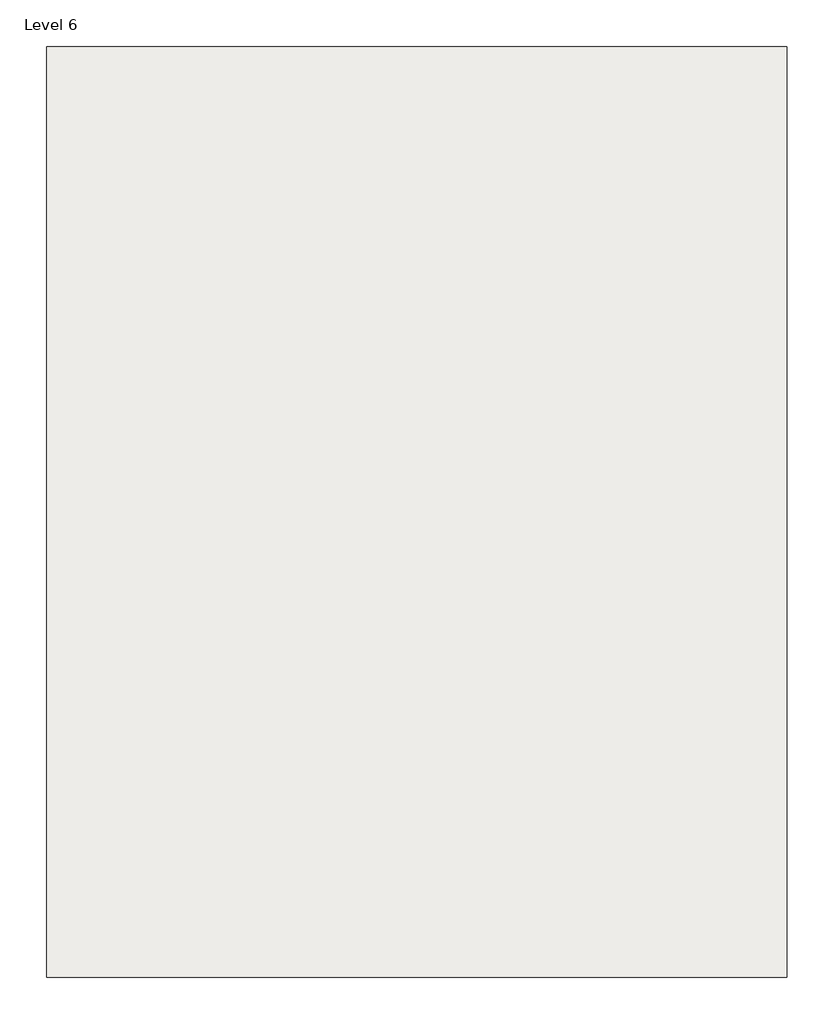
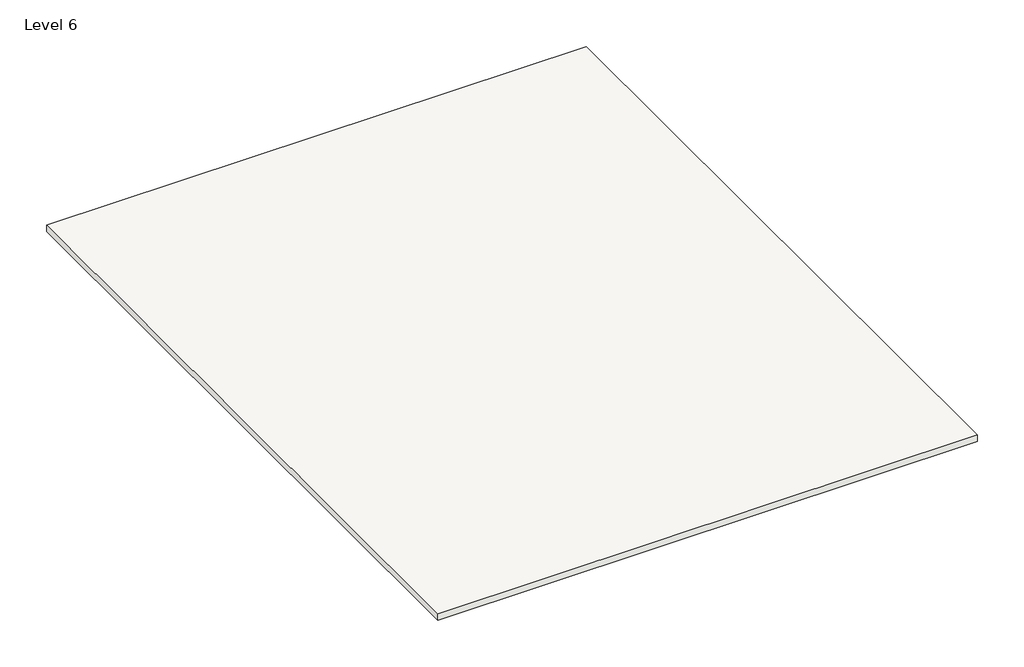
# One storey, incomplete: 1 roof.
"""IFC4 building model written with IfcOpenShell, lengths in millimetres."""

from ifc_helpers import new_model, si_unit, frame, origin, place, context, project, spatial, polyline, outline, extrude, element, save

model = new_model("IFC4")

# Units and contexts
model_context = context("Model", 3, world=origin())
ifc_project = project(units=[si_unit("LENGTHUNIT", "METRE", prefix="MILLI")], contexts=[model_context])

# Site, building, storey
site = spatial("IfcSite", under=ifc_project)
building = spatial("IfcBuilding", under=site)
storey = spatial("IfcBuildingStorey", under=building, Name="Level 6", Elevation=12801.6)

# Roof
placement = place(None, origin())
element("IfcRoof", 1, ObjectType="Generic - 12\"", at=placement, inside=storey, context=model_context, shape_type="SweptSolid", body=[
    extrude(outline(polyline([(-7200.0599931, 8005.7935985), (4687.1400069, 8005.7935985), (4687.1400069, -6929.4064015), (-7200.0599931, -6929.4064015), (-7200.0599931, 8005.7935985)])), frame((0.0, 0.0, 12649.2), z_axis=(0.0, 0.0, 1.0), x_axis=(1.0, 0.0, 0.0)), (0.0, 0.0, 1.0), 152.4),
])

save(model, "model.ifc")

# Revit data of these elements
# Type "Generic - 12\""
#   Assembly Code = "B1020"
#   Layers, outside or top first: 0' - 6" no material (function 1)
# Element 1 (IfcRoof, "Generic - 12\"")
#   built-in parameter 1001705 = 42 (stored number, unit not read)
#   built-in parameter 1001701 = -0.5 (stored number, unit not read)
#   built-in parameter 1001710 = 33615
#   Phase Created = New Construction
#   Materials on its faces: "Default Roof", "Oak Flooring"
# Materials
#   "Default Roof": colour RGB 88 101 114, transparency 0, Cost = 0
#   "Oak Flooring": class "Wood", colour RGB 216 169 114, transparency 0, Description = "Quercus Rubra", Cost = 0
